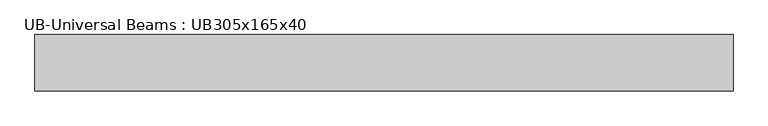
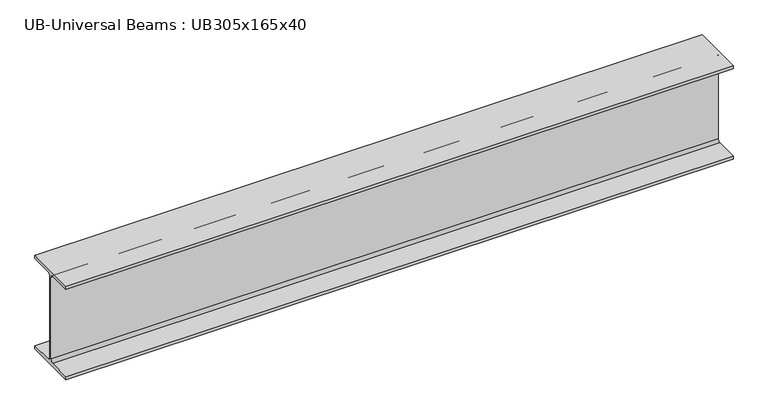
"""IFC4 building model written with IfcOpenShell, lengths in millimetres: beam geometry, UB-Universal Beams : UB305x165x40."""

from ifc_helpers import new_model, si_unit, point, frame, frame_2d, origin, place, context, project, spatial, polyline, circle_curve, trimmed, segment, composite_curve, outline, extrude, source, transform, mapped, element, save


def ub_universal_beams_ub305x165x40_f8f1f307(model_context):
    return source(origin(), model_context, "Body", "SweptSolid", [
        extrude(outline(composite_curve([segment(polyline([(82.5, -141.5), (82.5, -151.7), (-82.5, -151.7), (-82.5, -141.5), (-11.9, -141.5)]), True, "CONTINUOUS"), segment(trimmed(circle_curve(frame_2d((-11.9, -132.6)), 8.9), [point((-11.9, -141.5))], [point((-3.0, -132.6))], True, "CARTESIAN"), True, "CONTINUOUS"), segment(polyline([(-3.0, -132.6), (-3.0, 132.6)]), True, "CONTINUOUS"), segment(trimmed(circle_curve(frame_2d((-11.9, 132.6)), 8.9), [point((-3.0, 132.6))], [point((-11.9, 141.5))], True, "CARTESIAN"), True, "CONTINUOUS"), segment(polyline([(-11.9, 141.5), (-82.5, 141.5), (-82.5, 151.7), (82.5, 151.7), (82.5, 141.5), (11.9, 141.5)]), True, "CONTINUOUS"), segment(trimmed(circle_curve(frame_2d((11.9, 132.6)), 8.9), [point((11.9, 141.5))], [point((3.0, 132.6))], True, "CARTESIAN"), True, "CONTINUOUS"), segment(polyline([(3.0, 132.6), (3.0, -132.6)]), True, "CONTINUOUS"), segment(trimmed(circle_curve(frame_2d((11.9, -132.6)), 8.9), [point((3.0, -132.6))], [point((11.9, -141.5))], True, "CARTESIAN"), True, "CONTINUOUS"), segment(polyline([(11.9, -141.5), (82.5, -141.5)]), True, "CONTINUOUS")], self_intersect=False)), frame((-1084.2, 0.0, 0.0), z_axis=(1.0, 0.0, 0.0), x_axis=(0.0, 1.0, 0.0)), (0.0, 0.0, 1.0), 2047.0),
    ])


if __name__ == "__main__":
    model = new_model("IFC4")
    model_context = context("Model", 3, world=origin())
    ifc_project = project(units=[si_unit("LENGTHUNIT", "METRE", prefix="MILLI")], contexts=[model_context])
    site = spatial("IfcSite", under=ifc_project)
    building = spatial("IfcBuilding", under=site)
    placement = place(None, origin())
    ub_universal_beams_ub305x165x40_shape = ub_universal_beams_ub305x165x40_f8f1f307(model_context)
    element("IfcBeam", 1, ObjectType="UB-Universal Beams : UB305x165x40", at=placement, inside=building, context=model_context, shape_type="MappedRepresentation", body=[
        mapped(ub_universal_beams_ub305x165x40_shape, transform((0.0, 0.0, 0.0), x_axis=(1.0, 0.0, 0.0), y_axis=(0.0, 1.0, 0.0), z_axis=(0.0, 0.0, 1.0))),
    ])
    save(model, "model.ifc")

# Revit data of these elements
# Type "UB-Universal Beams : UB305x165x40"
#   Section Name Key = "UB305X165X40"
#   Width = 16.5 cm
#   Web Thickness = 0.6 cm
#   Web Fillet = 0.89 cm
#   Warping Constant = 164000.0 cm⁶
#   Torsional Moment of Inertia = 14.70 cm⁴
#   Section Area = 51.3 cm²
#   Plastic Modulus weak axis = 142.0 cm³
#   Plastic Modulus strong axis = 623.0 cm³
#   Nominal Weight = 40.2999 kgf/m
#   Moment of Inertia weak axis = 764.00 cm⁴
#   Moment of Inertia strong axis = 8503.00 cm⁴
#   Height = 30.34 cm
#   Flange Thickness = 1.02 cm
#   Elastic Modulus weak axis = 92.6 cm³
#   Elastic Modulus strong axis = 560.0 cm³
#   Centroid Vertical = 15.17 cm
#   Centroid Horizontal = 8.25 cm
#   Bolt Spacing = 9.0 cm
#   Length [instance default] = 1500 mm
#   Structural Material [instance default] = Metal - Steel 43-275
#   Type Comments = ""
#   Assembly Code = ""
# Element 1 (IfcBeam, "UB-Universal Beams : UB305x165x40")
#   Materials on its faces: "Metal - Steel 43-275"
# Materials
#   "Metal - Steel 43-275": class "Metal", colour RGB 247 247 247, transparency 0, Cost = 0
